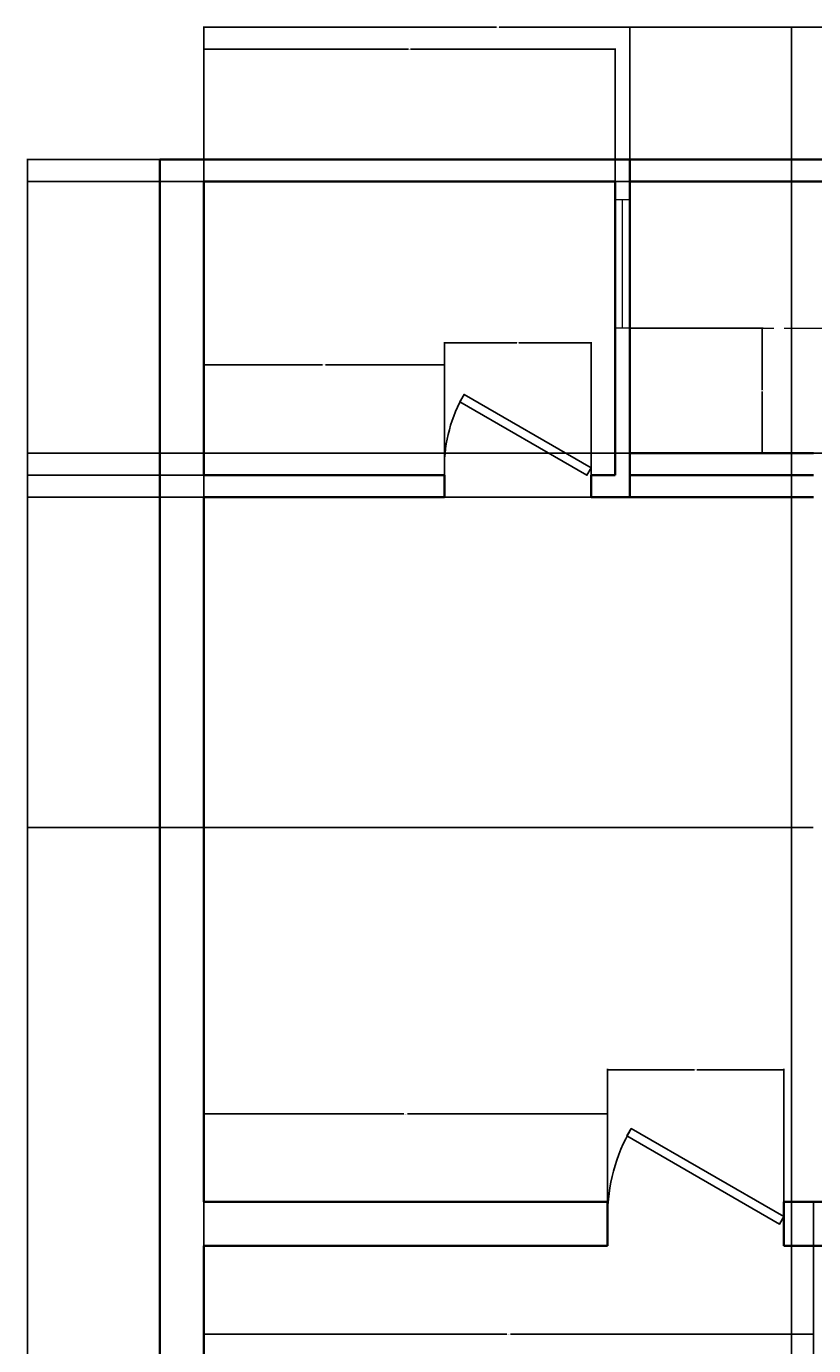
# Model space of a CAD drawing. Units: inches. Extents: x 2599 to 2953, y 557 to 1152.
# Tile 6 of 7: x 2599 to 2759, y 882 to 1152. Entities that reach past the tile are written whole.
import ezdxf

# ---------------------------------------------------------------- set-up
doc = ezdxf.new("R2010")
doc.units = ezdxf.units.IN
doc.linetypes.add('ACAD_ISO02W100', pattern=[15, 12, -3])
for name, color, linetype, lineweight in [('A-ANNO-DIMS', 2, 'Continuous', 18), ('A-DOOR', 4, 'Continuous', 25), ('A-GLAZ', 4, 'Continuous', 18), ('A-WALL', 7, 'Continuous', 35), ('A-WALL-OVHD', 8, 'ACAD_ISO02W100', 18)]:
    doc.layers.add(name, color=color, linetype=linetype, lineweight=lineweight)
doc.styles.get("Standard").update_dxf_attribs({"font": 'arial.ttf'})
doc.dimstyles.get("Standard").update_dxf_attribs({"dimtxt": 0.18, "dimasz": 0.18, "dimexe": 0.18, "dimexo": 0.0625, "dimgap": 0.09, "dimtad": 0, "dimtih": 1, "dimtoh": 1, "dimdec": 4, "dimzin": 0, "dimdsep": 46, "dimtxsty": 'Standard', "dimcen": 0.09, "dimadec": 0, "dimazin": 0, "dimtfac": 1, "dimtdec": 4, "dimtofl": 0, "dimtmove": 0, "dimatfit": 3, "dimfxl": 1, "dimtolj": 1, "dimtzin": 0, "dimarcsym": 0})

# ---------------------------------------------------------------- blocks, each defined once
blk = doc.blocks.new('*U3')
for p, q in [((-30, 0), (-30, -6)), ((0, 0), (0, -6))]:
    blk.add_line(p, q)
blk.add_lwpolyline([(0, 0), (-25.98, 15), (-26.86, 13.48), (-0.88, -1.52)], close=True)
blk.add_arc((0, 0), 30, 150, 180)
blk = doc.blocks.new('*U7')
for p, q in [((0, 0), (0, -6)), ((-36, 0), (-36, -6))]:
    blk.add_line(p, q)
blk.add_lwpolyline([(0, 0), (-31.18, 18), (-32.05, 16.48), (-0.88, -1.52)], close=True)
blk.add_arc((0, 0), 36, 150, 180)
blk = doc.blocks.new('WIN-26_335IN')
for p, q in [((0, 26.33), (3, 26.33)), ((1.5, 0), (1.5, 26.33)), ((3, 0), (0, 0))]:
    blk.add_line(p, q)
blk = doc.blocks.new('*D21')
at = {"layer": 'A-ANNO-DIMS', "color": 0, "lineweight": -2, "transparency": 16777216}
for p, q in [((2625.92, 1124.28), (2625.92, 557.16)), ((2925.92, 584.28), (2925.92, 557.16)), ((2626.1, 557.34), (2775.63, 557.34)), ((2925.74, 557.34), (2776.21, 557.34))]:
    blk.add_line(p, q, dxfattribs=at)
at = {"layer": 'A-ANNO-DIMS', "color": 0, "transparency": 16777216}
for points in [[(2626.1, 557.37), (2626.1, 557.31), (2625.92, 557.34)], [(2925.74, 557.37), (2925.74, 557.31), (2925.92, 557.34)]]:
    blk.add_solid(points, dxfattribs=at)
at = {"layer": 'Defpoints', "color": 0, "transparency": 16777216}
for p in [(2625.92, 1124.34), (2925.92, 584.34), (2925.92, 557.34)]:
    blk.add_point(p, dxfattribs=at)
at = {"layer": 'A-ANNO-DIMS', "color": 0, "transparency": 16777216, "insert": (2775.92, 557.34), "char_height": 0.18, "attachment_point": 5}
blk.add_mtext('\\A1;300', dxfattribs=at)
blk = doc.blocks.new('*D22')
at = {"layer": 'A-ANNO-DIMS', "color": 0, "lineweight": -2, "transparency": 16777216}
for p, q in [((2625.86, 1124.34), (2598.74, 1124.34)), ((2598.92, 1124.16), (2598.92, 854.52)), ((2598.92, 584.52), (2598.92, 854.16)), ((2625.86, 584.34), (2598.74, 584.34))]:
    blk.add_line(p, q, dxfattribs=at)
at = {"layer": 'A-ANNO-DIMS', "color": 0, "transparency": 16777216}
for points in [[(2598.89, 1124.16), (2598.95, 1124.16), (2598.92, 1124.34)], [(2598.89, 584.52), (2598.95, 584.52), (2598.92, 584.34)]]:
    blk.add_solid(points, dxfattribs=at)
at = {"layer": 'Defpoints', "color": 0, "transparency": 16777216}
for p in [(2598.92, 1124.34), (2625.92, 1124.34), (2625.92, 584.34)]:
    blk.add_point(p, dxfattribs=at)
at = {"layer": 'A-ANNO-DIMS', "color": 0, "transparency": 16777216, "insert": (2598.92, 854.34), "char_height": 0.18, "attachment_point": 5}
blk.add_mtext('\\A1;540', dxfattribs=at)
blk = doc.blocks.new('*D37')
at = {"layer": 'A-ANNO-DIMS', "color": 0, "lineweight": -2, "transparency": 16777216}
for p, q in [((2634.92, 761.4), (2634.92, 1151.53)), ((2635.1, 1151.35), (2694.64, 1151.35)), ((2754.74, 1151.35), (2695.2, 1151.35)), ((2754.92, 761.4), (2754.92, 1151.53))]:
    blk.add_line(p, q, dxfattribs=at)
at = {"layer": 'A-ANNO-DIMS', "color": 0, "transparency": 16777216}
for points in [[(2635.1, 1151.38), (2635.1, 1151.32), (2634.92, 1151.35)], [(2754.74, 1151.38), (2754.74, 1151.32), (2754.92, 1151.35)]]:
    blk.add_solid(points, dxfattribs=at)
at = {"layer": 'Defpoints', "color": 0, "transparency": 16777216}
for p in [(2754.92, 1151.35), (2634.92, 761.34), (2754.92, 761.34)]:
    blk.add_point(p, dxfattribs=at)
at = {"layer": 'A-ANNO-DIMS', "color": 0, "transparency": 16777216, "insert": (2694.92, 1151.35), "char_height": 0.18, "attachment_point": 5}
blk.add_mtext('\\A1;120', dxfattribs=at)
blk = doc.blocks.new('*D54')
at = {"layer": 'A-ANNO-DIMS', "color": 0, "lineweight": -2, "transparency": 16777216}
for p, q in [((2634.92, 911.28), (2634.92, 884.16)), ((2759.42, 911.28), (2759.42, 884.16)), ((2635.1, 884.34), (2696.79, 884.34)), ((2759.24, 884.34), (2697.56, 884.34))]:
    blk.add_line(p, q, dxfattribs=at)
at = {"layer": 'A-ANNO-DIMS', "color": 0, "transparency": 16777216}
for points in [[(2635.1, 884.37), (2635.1, 884.31), (2634.92, 884.34)], [(2759.24, 884.37), (2759.24, 884.31), (2759.42, 884.34)]]:
    blk.add_solid(points, dxfattribs=at)
at = {"layer": 'Defpoints', "color": 0, "transparency": 16777216}
for p in [(2634.92, 911.34), (2759.42, 911.34), (2634.92, 884.34)]:
    blk.add_point(p, dxfattribs=at)
at = {"layer": 'A-ANNO-DIMS', "color": 0, "transparency": 16777216, "insert": (2697.17, 884.34), "char_height": 0.18, "attachment_point": 5}
blk.add_mtext('\\A1;124.5', dxfattribs=at)
blk = doc.blocks.new('*D55')
at = {"layer": 'A-ANNO-DIMS', "color": 0, "lineweight": -2, "transparency": 16777216}
for p, q in [((2759.42, 911.28), (2759.42, 557.16)), ((2787.92, 911.28), (2787.92, 557.16)), ((2759.6, 557.34), (2773.35, 557.34)), ((2787.74, 557.34), (2774, 557.34))]:
    blk.add_line(p, q, dxfattribs=at)
at = {"layer": 'A-ANNO-DIMS', "color": 0, "transparency": 16777216}
for points in [[(2759.6, 557.37), (2759.6, 557.31), (2759.42, 557.34)], [(2787.74, 557.37), (2787.74, 557.31), (2787.92, 557.34)]]:
    blk.add_solid(points, dxfattribs=at)
at = {"layer": 'Defpoints', "color": 0, "transparency": 16777216}
for p in [(2759.42, 911.34), (2787.92, 911.34), (2787.92, 557.34)]:
    blk.add_point(p, dxfattribs=at)
at = {"layer": 'A-ANNO-DIMS', "color": 0, "transparency": 16777216, "insert": (2773.67, 557.34), "char_height": 0.18, "attachment_point": 5}
blk.add_mtext('\\A1;28.5', dxfattribs=at)
blk = doc.blocks.new('*D58')
at = {"layer": 'A-ANNO-DIMS', "color": 0, "lineweight": -2, "transparency": 16777216}
for p, q in [((2634.92, 1119.9), (2634.92, 1147.03)), ((2635.1, 1146.85), (2676.7, 1146.85)), ((2718.74, 1146.85), (2677.14, 1146.85)), ((2718.92, 1119.9), (2718.92, 1147.03))]:
    blk.add_line(p, q, dxfattribs=at)
at = {"layer": 'A-ANNO-DIMS', "color": 0, "transparency": 16777216}
for points in [[(2635.1, 1146.88), (2635.1, 1146.82), (2634.92, 1146.85)], [(2718.74, 1146.88), (2718.74, 1146.82), (2718.92, 1146.85)]]:
    blk.add_solid(points, dxfattribs=at)
at = {"layer": 'Defpoints', "color": 0, "transparency": 16777216}
for p in [(2718.92, 1146.85), (2634.92, 1119.84), (2718.92, 1119.84)]:
    blk.add_point(p, dxfattribs=at)
at = {"layer": 'A-ANNO-DIMS', "color": 0, "transparency": 16777216, "insert": (2676.92, 1146.85), "char_height": 0.18, "attachment_point": 5}
blk.add_mtext('\\A1;84', dxfattribs=at)
blk = doc.blocks.new('*D59')
at = {"layer": 'A-ANNO-DIMS', "color": 0, "lineweight": -2, "transparency": 16777216}
for p, q in [((2721.92, 1124.4), (2721.92, 1151.53)), ((2722.1, 1151.35), (2775.64, 1151.35)), ((2829.74, 1151.35), (2776.2, 1151.35)), ((2829.92, 1124.4), (2829.92, 1151.53))]:
    blk.add_line(p, q, dxfattribs=at)
at = {"layer": 'A-ANNO-DIMS', "color": 0, "transparency": 16777216}
for points in [[(2722.1, 1151.38), (2722.1, 1151.32), (2721.92, 1151.35)], [(2829.74, 1151.38), (2829.74, 1151.32), (2829.92, 1151.35)]]:
    blk.add_solid(points, dxfattribs=at)
at = {"layer": 'Defpoints', "color": 0, "transparency": 16777216}
for p in [(2829.92, 1151.35), (2721.92, 1124.34), (2829.92, 1124.34)]:
    blk.add_point(p, dxfattribs=at)
at = {"layer": 'A-ANNO-DIMS', "color": 0, "transparency": 16777216, "insert": (2775.92, 1151.35), "char_height": 0.18, "attachment_point": 5}
blk.add_mtext('\\A1;108', dxfattribs=at)
blk = doc.blocks.new('*D61')
at = {"layer": 'A-ANNO-DIMS', "color": 0, "lineweight": -2, "transparency": 16777216}
for p, q in [((2634.86, 1119.84), (2598.74, 1119.84)), ((2598.92, 1119.66), (2598.92, 1090.02)), ((2598.92, 1060.02), (2598.92, 1089.66)), ((2634.86, 1059.84), (2598.74, 1059.84))]:
    blk.add_line(p, q, dxfattribs=at)
at = {"layer": 'A-ANNO-DIMS', "color": 0, "transparency": 16777216}
for points in [[(2598.89, 1119.66), (2598.95, 1119.66), (2598.92, 1119.84)], [(2598.89, 1060.02), (2598.95, 1060.02), (2598.92, 1059.84)]]:
    blk.add_solid(points, dxfattribs=at)
at = {"layer": 'Defpoints', "color": 0, "transparency": 16777216}
for p in [(2598.92, 1119.84), (2634.92, 1119.84), (2634.92, 1059.84)]:
    blk.add_point(p, dxfattribs=at)
at = {"layer": 'A-ANNO-DIMS', "color": 0, "transparency": 16777216, "insert": (2598.92, 1089.84), "char_height": 0.18, "attachment_point": 5}
blk.add_mtext('\\A1;60', dxfattribs=at)
blk = doc.blocks.new('*D62')
at = {"layer": 'A-ANNO-DIMS', "color": 0, "lineweight": -2, "transparency": 16777216}
for p, q in [((2634.92, 1055.4), (2634.92, 1082.53)), ((2635.1, 1082.35), (2659.16, 1082.35)), ((2683.84, 1082.35), (2659.78, 1082.35)), ((2684.02, 1055.4), (2684.02, 1082.53))]:
    blk.add_line(p, q, dxfattribs=at)
at = {"layer": 'A-ANNO-DIMS', "color": 0, "transparency": 16777216}
for points in [[(2635.1, 1082.38), (2635.1, 1082.32), (2634.92, 1082.35)], [(2683.84, 1082.38), (2683.84, 1082.32), (2684.02, 1082.35)]]:
    blk.add_solid(points, dxfattribs=at)
at = {"layer": 'Defpoints', "color": 0, "transparency": 16777216}
for p in [(2684.02, 1082.35), (2634.92, 1055.34), (2684.02, 1055.34)]:
    blk.add_point(p, dxfattribs=at)
at = {"layer": 'A-ANNO-DIMS', "color": 0, "transparency": 16777216, "insert": (2659.47, 1082.35), "char_height": 0.18, "attachment_point": 5}
blk.add_mtext('\\A1;49.1', dxfattribs=at)
blk = doc.blocks.new('*D63')
at = {"layer": 'A-ANNO-DIMS', "color": 0, "lineweight": -2, "transparency": 16777216}
for p, q in [((2684.02, 1059.9), (2684.02, 1087.03)), ((2684.2, 1086.85), (2698.8, 1086.85)), ((2713.84, 1086.85), (2699.24, 1086.85)), ((2714.02, 1059.9), (2714.02, 1087.03))]:
    blk.add_line(p, q, dxfattribs=at)
at = {"layer": 'A-ANNO-DIMS', "color": 0, "transparency": 16777216}
for points in [[(2684.2, 1086.88), (2684.2, 1086.82), (2684.02, 1086.85)], [(2713.84, 1086.88), (2713.84, 1086.82), (2714.02, 1086.85)]]:
    blk.add_solid(points, dxfattribs=at)
at = {"layer": 'Defpoints', "color": 0, "transparency": 16777216}
for p in [(2714.02, 1086.85), (2684.02, 1059.84), (2714.02, 1059.84)]:
    blk.add_point(p, dxfattribs=at)
at = {"layer": 'A-ANNO-DIMS', "color": 0, "transparency": 16777216, "insert": (2699.02, 1086.85), "char_height": 0.18, "attachment_point": 5}
blk.add_mtext('\\A1;30', dxfattribs=at)
blk = doc.blocks.new('*D66')
at = {"layer": 'A-ANNO-DIMS', "color": 0, "lineweight": -2, "transparency": 16777216}
for p, q in [((2634.92, 902.4), (2634.92, 929.53)), ((2635.1, 929.35), (2675.74, 929.35)), ((2717.17, 929.35), (2676.53, 929.35)), ((2717.35, 902.4), (2717.35, 929.53))]:
    blk.add_line(p, q, dxfattribs=at)
at = {"layer": 'A-ANNO-DIMS', "color": 0, "transparency": 16777216}
for points in [[(2635.1, 929.38), (2635.1, 929.32), (2634.92, 929.35)], [(2717.17, 929.38), (2717.17, 929.32), (2717.35, 929.35)]]:
    blk.add_solid(points, dxfattribs=at)
at = {"layer": 'Defpoints', "color": 0, "transparency": 16777216}
for p in [(2717.35, 929.35), (2634.92, 902.34), (2717.35, 902.34)]:
    blk.add_point(p, dxfattribs=at)
at = {"layer": 'A-ANNO-DIMS', "color": 0, "transparency": 16777216, "insert": (2676.14, 929.35), "char_height": 0.18, "attachment_point": 5}
blk.add_mtext('\\A1;82.43', dxfattribs=at)
blk = doc.blocks.new('*D67')
at = {"layer": 'A-ANNO-DIMS', "color": 0, "lineweight": -2, "transparency": 16777216}
for p, q in [((2717.35, 911.4), (2717.35, 938.53)), ((2717.53, 938.35), (2735.13, 938.35)), ((2753.17, 938.35), (2735.57, 938.35)), ((2753.35, 911.4), (2753.35, 938.53))]:
    blk.add_line(p, q, dxfattribs=at)
at = {"layer": 'A-ANNO-DIMS', "color": 0, "transparency": 16777216}
for points in [[(2717.53, 938.38), (2717.53, 938.32), (2717.35, 938.35)], [(2753.17, 938.38), (2753.17, 938.32), (2753.35, 938.35)]]:
    blk.add_solid(points, dxfattribs=at)
at = {"layer": 'Defpoints', "color": 0, "transparency": 16777216}
for p in [(2753.35, 938.35), (2717.35, 911.34), (2753.35, 911.34)]:
    blk.add_point(p, dxfattribs=at)
at = {"layer": 'A-ANNO-DIMS', "color": 0, "transparency": 16777216, "insert": (2735.35, 938.35), "char_height": 0.18, "attachment_point": 5}
blk.add_mtext('\\A1;36', dxfattribs=at)
blk = doc.blocks.new('*D70')
at = {"layer": 'A-ANNO-DIMS', "color": 0, "lineweight": -2, "transparency": 16777216}
for p, q in [((2759.36, 1055.34), (2598.74, 1055.34)), ((2598.92, 1055.16), (2598.92, 1021.77)), ((2598.92, 988.02), (2598.92, 1021.41)), ((2759.36, 987.84), (2598.74, 987.84))]:
    blk.add_line(p, q, dxfattribs=at)
at = {"layer": 'A-ANNO-DIMS', "color": 0, "transparency": 16777216}
for points in [[(2598.89, 1055.16), (2598.95, 1055.16), (2598.92, 1055.34)], [(2598.89, 988.02), (2598.95, 988.02), (2598.92, 987.84)]]:
    blk.add_solid(points, dxfattribs=at)
at = {"layer": 'Defpoints', "color": 0, "transparency": 16777216}
for p in [(2598.92, 1055.34), (2759.42, 1055.34), (2759.42, 987.84)]:
    blk.add_point(p, dxfattribs=at)
at = {"layer": 'A-ANNO-DIMS', "color": 0, "transparency": 16777216, "insert": (2598.92, 1021.59), "char_height": 0.18, "attachment_point": 5}
blk.add_mtext('\\A1;67.5', dxfattribs=at)
blk = doc.blocks.new('*D71')
at = {"layer": 'A-ANNO-DIMS', "color": 0, "lineweight": -2, "transparency": 16777216}
for p, q in [((2829.86, 1119.84), (2598.74, 1119.84)), ((2598.92, 1119.66), (2598.92, 1092.27)), ((2598.92, 1064.52), (2598.92, 1091.91)), ((2787.86, 1064.34), (2598.74, 1064.34))]:
    blk.add_line(p, q, dxfattribs=at)
at = {"layer": 'A-ANNO-DIMS', "color": 0, "transparency": 16777216}
for points in [[(2598.89, 1119.66), (2598.95, 1119.66), (2598.92, 1119.84)], [(2598.89, 1064.52), (2598.95, 1064.52), (2598.92, 1064.34)]]:
    blk.add_solid(points, dxfattribs=at)
at = {"layer": 'Defpoints', "color": 0, "transparency": 16777216}
for p in [(2598.92, 1119.84), (2829.92, 1119.84), (2787.92, 1064.34)]:
    blk.add_point(p, dxfattribs=at)
at = {"layer": 'A-ANNO-DIMS', "color": 0, "transparency": 16777216, "insert": (2598.92, 1092.09), "char_height": 0.18, "attachment_point": 5}
blk.add_mtext('\\A1;55.5', dxfattribs=at)
blk = doc.blocks.new('*D72')
at = {"layer": 'A-ANNO-DIMS', "color": 0, "lineweight": -2, "transparency": 16777216}
for p, q in [((2721.98, 1089.84), (2749.1, 1089.84)), ((2748.92, 1089.66), (2748.92, 1077.27)), ((2748.92, 1064.52), (2748.92, 1076.91)), ((2721.98, 1064.34), (2749.1, 1064.34))]:
    blk.add_line(p, q, dxfattribs=at)
at = {"layer": 'A-ANNO-DIMS', "color": 0, "transparency": 16777216}
for points in [[(2748.89, 1089.66), (2748.95, 1089.66), (2748.92, 1089.84)], [(2748.89, 1064.52), (2748.95, 1064.52), (2748.92, 1064.34)]]:
    blk.add_solid(points, dxfattribs=at)
at = {"layer": 'Defpoints', "color": 0, "transparency": 16777216}
for p in [(2721.92, 1089.84), (2721.92, 1064.34), (2748.92, 1064.34)]:
    blk.add_point(p, dxfattribs=at)
at = {"layer": 'A-ANNO-DIMS', "color": 0, "transparency": 16777216, "insert": (2748.92, 1077.09), "char_height": 0.18, "attachment_point": 5}
blk.add_mtext('\\A1;25.5', dxfattribs=at)

msp = doc.modelspace()

# ---------------------------------------------------------------- linework, layer by layer
at = {"layer": 'A-WALL'}
for p, q in [((2625.9211, 1124.3417), (2625.9211, 584.3417)), ((2721.9211, 1124.3417), (2625.9211, 1124.3417)), ((2721.9211, 1124.3417), (2721.9211, 1055.3417)), ((2721.9211, 1124.3417), (2829.9211, 1124.3417)), ((2634.9211, 1119.8417), (2634.9211, 1059.8417)), ((2718.9211, 1119.8417), (2634.9211, 1119.8417)), ((2718.9211, 1119.8417), (2718.9211, 1059.8417)), ((2829.9211, 1119.8417), (2721.9211, 1119.8417)), ((2759.4211, 1064.3417), (2721.9211, 1064.3417)), ((2684.019, 1059.8417), (2634.9211, 1059.8417)), ((2684.019, 1059.8417), (2684.019, 1055.3417)), ((2718.9211, 1059.8417), (2714.019, 1059.8417)), ((2714.019, 1059.8417), (2714.019, 1055.3417)), ((2759.4211, 1059.8417), (2721.9211, 1059.8417)), ((2634.9211, 1055.3417), (2634.9211, 911.3417)), ((2684.019, 1055.3417), (2634.9211, 1055.3417)), ((2721.9211, 1055.3417), (2714.019, 1055.3417)), ((2759.4211, 1055.3417), (2721.9211, 1055.3417)), ((2717.3499, 911.3417), (2634.9211, 911.3417)), ((2717.3499, 911.3417), (2717.3499, 902.3417)), ((2753.3499, 911.3417), (2753.3499, 902.3417)), ((2783.4211, 911.3417), (2753.3499, 911.3417)), ((2634.9211, 902.3417), (2634.9211, 770.3417)), ((2717.3499, 902.3417), (2634.9211, 902.3417)), ((2795.4243, 902.3417), (2753.3499, 902.3417))]:
    msp.add_line(p, q, dxfattribs=at)
at = {"layer": 'A-WALL-OVHD', "ltscale": 0.7}
msp.add_line((2721.9211, 1089.8417), (2829.9211, 1089.8417), dxfattribs=at)

# ---------------------------------------------------------------- block references
at = {"layer": 'A-DOOR'}
for name, p in [('*U3', (2714.019, 1061.3417)), ('*U7', (2753.3499, 908.3417))]:
    msp.add_blockref(name, p, dxfattribs=at)
at = {"layer": 'A-GLAZ'}
msp.add_blockref('WIN-26_335IN', (2718.921, 1089.842), dxfattribs=at)

# ---------------------------------------------------------------- dimensions: what is measured, and where the dimension line sits
at = {"layer": 'A-ANNO-DIMS'}
for base, p1, p2, override, picture, middle in [((2754.9211, 1151.3452), (2634.9211, 761.3417), (2754.9211, 761.3417), {"dimdec": 0, "dimlfac": 1, "dimrnd": 0, "dimzin": 0, "dimdsep": 46, "dimlunit": 2}, '*D37', (2694.9211, 1151.3452)), ((2829.9211, 1151.3452), (2721.9211, 1124.3417), (2829.9211, 1124.3417), {"dimdec": 0, "dimlfac": 1, "dimrnd": 0, "dimzin": 0, "dimdsep": 46, "dimlunit": 2}, '*D59', (2775.9211, 1151.3452)), ((2718.9211, 1146.8452), (2634.9211, 1119.8417), (2718.9211, 1119.8417), {"dimdec": 0, "dimlfac": 1, "dimrnd": 0, "dimzin": 0, "dimdsep": 46, "dimlunit": 2}, '*D58', (2676.9211, 1146.8452)), ((2925.9211, 557.3382), (2625.9211, 1124.3417), (2925.9211, 584.3417), {"dimdec": 0, "dimlfac": 1, "dimrnd": 0, "dimzin": 0, "dimdsep": 46, "dimlunit": 2}, '*D21', (2775.9211, 557.3382)), ((2714.019, 1086.8452), (2684.019, 1059.8417), (2714.019, 1059.8417), {"dimdec": 0, "dimlfac": 1, "dimrnd": 0, "dimzin": 0, "dimdsep": 46, "dimlunit": 2}, '*D63', (2699.019, 1086.8452)), ((2684.019, 1082.3452), (2634.9211, 1055.3417), (2684.019, 1055.3417), {"dimdec": 1, "dimlfac": 1, "dimrnd": 0, "dimzin": 0, "dimdsep": 46, "dimlunit": 2}, '*D62', (2659.4701, 1082.3452)), ((2753.3499, 938.3452), (2717.3499, 911.3417), (2753.3499, 911.3417), {"dimdec": 0, "dimlfac": 1, "dimrnd": 0, "dimzin": 0, "dimdsep": 46, "dimlunit": 2}, '*D67', (2735.3499, 938.3452)), ((2717.3499, 929.3452), (2634.9211, 902.3417), (2717.3499, 902.3417), {"dimdec": 2, "dimlfac": 1, "dimrnd": 0, "dimzin": 0, "dimdsep": 46, "dimlunit": 2}, '*D66', (2676.1355, 929.3452)), ((2787.9211, 557.3382), (2759.4211, 911.3417), (2787.9211, 911.3417), {"dimdec": 1, "dimlfac": 1, "dimrnd": 0, "dimzin": 0, "dimdsep": 46, "dimlunit": 2}, '*D55', (2773.6711, 557.3382))]:
    dim = msp.add_linear_dim(base=base, p1=p1, p2=p2, dimstyle='Standard', override=override, dxfattribs=at)
    dim.commit()
    dim.dimension.update_dxf_attribs({"geometry": picture, "text_midpoint": middle})
for base, p1, p2, angle, override, picture, middle in [((2598.9176, 1124.3417), (2625.9211, 584.3417), (2625.9211, 1124.3417), 90, {"dimdec": 0, "dimlfac": 1, "dimrnd": 0, "dimzin": 0, "dimdsep": 46, "dimlunit": 2}, '*D22', (2598.9176, 854.3417)), ((2598.9176, 1119.8417), (2787.9211, 1064.3417), (2829.9211, 1119.8417), 90, {"dimdec": 1, "dimlfac": 1, "dimrnd": 0, "dimzin": 0, "dimdsep": 46, "dimlunit": 2}, '*D71', (2598.9176, 1092.0917)), ((2598.9176, 1119.8417), (2634.9211, 1059.8417), (2634.9211, 1119.8417), 90, {"dimdec": 0, "dimlfac": 1, "dimrnd": 0, "dimzin": 0, "dimdsep": 46, "dimlunit": 2}, '*D61', (2598.9176, 1089.8417)), ((2748.9246, 1064.3417), (2721.9211, 1089.8417), (2721.9211, 1064.3417), 270, {"dimdec": 1, "dimlfac": 1, "dimrnd": 0, "dimzin": 0, "dimdsep": 46, "dimlunit": 2}, '*D72', (2748.9246, 1077.0917)), ((2598.9176, 1055.3417), (2759.4211, 987.8417), (2759.4211, 1055.3417), 90, {"dimdec": 1, "dimlfac": 1, "dimrnd": 0, "dimzin": 0, "dimdsep": 46, "dimlunit": 2}, '*D70', (2598.9176, 1021.5917)), ((2634.9211, 884.3382), (2759.4211, 911.3417), (2634.9211, 911.3417), 180, {"dimdec": 1, "dimlfac": 1, "dimrnd": 0, "dimzin": 0, "dimdsep": 46, "dimlunit": 2}, '*D54', (2697.1711, 884.3382))]:
    dim = msp.add_linear_dim(base=base, p1=p1, p2=p2, angle=angle, dimstyle='Standard', override=override, dxfattribs=at)
    dim.commit()
    dim.dimension.update_dxf_attribs({"geometry": picture, "text_midpoint": middle})

doc.saveas('drawing.dxf')
